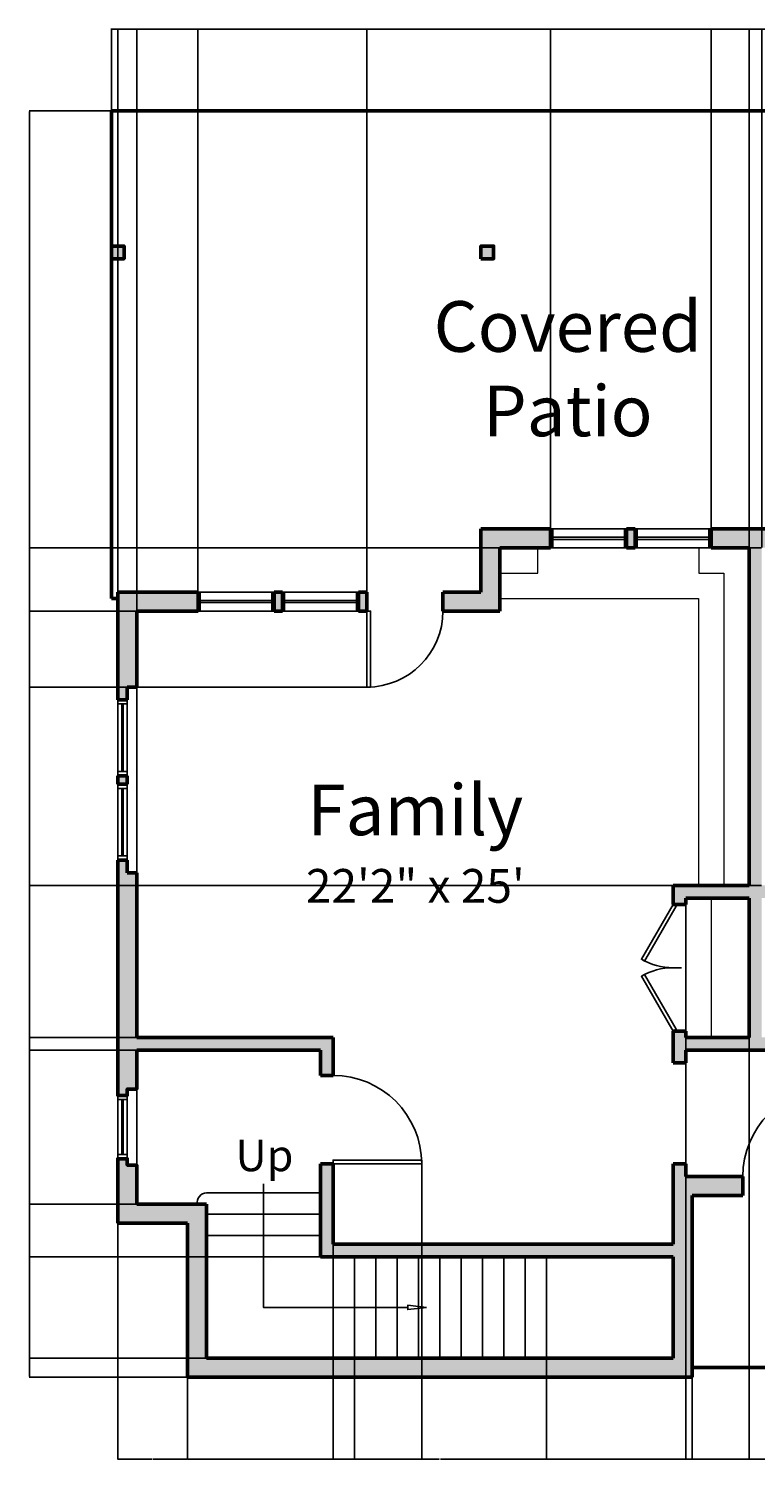
# Model space of a CAD drawing. Units: inches. Extents: x 296 to 2116, y 330 to 1460.
# Tile 7 of 9: x 1276 to 1620, y 779 to 1457. Entities that reach past the tile are written whole.
import ezdxf

# ---------------------------------------------------------------- set-up
doc = ezdxf.new("R2010")
doc.units = ezdxf.units.IN
for name, color, linetype, lineweight in [('A-ANNO-DIMS', 2, 'Continuous', 18), ('A-ANNO-TEXT', 7, 'Continuous', 18), ('A-AREA-IDEN', 7, 'Continuous', 25), ('A-DOOR', 3, 'Continuous', 25), ('A-FLOR-FIXT', 8, 'Continuous', 18), ('A-FLOR-STRS', 40, 'Continuous', 25), ('A-GLAZ', 4, 'Continuous', 25), ('A-WALL', 7, 'Continuous', 50), ('A-WALL-PATT', 8, 'Continuous', 13)]:
    doc.layers.add(name, color=color, linetype=linetype, lineweight=lineweight)
doc.styles.get("Standard").update_dxf_attribs({"font": 'arial.ttf'})
doc.dimstyles.get("Standard").update_dxf_attribs({"dimtxt": 0.18, "dimasz": 0.18, "dimexe": 0.18, "dimexo": 0.0625, "dimgap": 0.09, "dimtad": 0, "dimtih": 1, "dimtoh": 1, "dimdec": 4, "dimzin": 0, "dimdsep": 46, "dimtxsty": 'Standard', "dimcen": 0.09, "dimadec": 0, "dimazin": 0, "dimtfac": 1, "dimtdec": 4, "dimtofl": 0, "dimtmove": 0, "dimatfit": 3, "dimfxl": 1, "dimtolj": 1, "dimtzin": 0, "dimarcsym": 0})

# ---------------------------------------------------------------- blocks, each defined once
blk = doc.blocks.new('*U22')
for p, q in [((0, 0), (0, 4)), ((36, 0), (36, 4))]:
    blk.add_line(p, q)
blk.add_lwpolyline([(0, 0), (0, -36), (1.75, -36), (1.75, 0)], close=True)
blk.add_arc((0, 0), 36, 270, 0)
blk = doc.blocks.new('*U23')
for p, q in [((-40, 0), (-40, -4)), ((0, 0), (0, -4))]:
    blk.add_line(p, q)
blk.add_lwpolyline([(0, 0), (0, 40), (-1.75, 40), (-1.75, 0)], close=True)
blk.add_arc((0, 0), 40, 90, 180)
blk = doc.blocks.new('*U26')
for p, q in [((-30, 0), (-30, 4)), ((0, 0), (0, 4))]:
    blk.add_line(p, q)
blk.add_lwpolyline([(0, 0), (-25.98, -15), (-26.86, -13.48), (-0.88, 1.52)], close=True)
blk.add_arc((0, 0), 30, 180, 210)
blk = doc.blocks.new('*D67')
at = {"layer": 'A-ANNO-DIMS', "color": 0, "lineweight": -2, "transparency": 16777216}
for p, q in [((1315.18, 1418.02), (1315.18, 1456.98)), ((1315.36, 1456.8), (1695.9, 1456.8)), ((2077, 1456.8), (1696.47, 1456.8)), ((2077.18, 1408.02), (2077.18, 1456.98))]:
    blk.add_line(p, q, dxfattribs=at)
at = {"layer": 'A-ANNO-DIMS', "color": 0, "transparency": 16777216}
for points in [[(1315.36, 1456.83), (1315.36, 1456.77), (1315.18, 1456.8)], [(2077, 1456.83), (2077, 1456.77), (2077.18, 1456.8)]]:
    blk.add_solid(points, dxfattribs=at)
at = {"layer": 'Defpoints', "color": 0, "transparency": 16777216}
for p in [(2077.18, 1456.8), (1315.18, 1417.95), (2077.18, 1407.95)]:
    blk.add_point(p, dxfattribs=at)
at = {"layer": 'A-ANNO-DIMS', "color": 0, "transparency": 16777216, "insert": (1696.18, 1456.8), "char_height": 0.18, "attachment_point": 5}
blk.add_mtext('\\A1;762', dxfattribs=at)
blk = doc.blocks.new('*D68')
at = {"layer": 'A-ANNO-DIMS', "color": 0, "lineweight": -2, "transparency": 16777216}
for p, q in [((1315.12, 1417.95), (1276.15, 1417.95)), ((1276.33, 1417.77), (1276.33, 1118.16)), ((1276.33, 818.18), (1276.33, 1117.79)), ((1351.12, 818), (1276.15, 818))]:
    blk.add_line(p, q, dxfattribs=at)
at = {"layer": 'A-ANNO-DIMS', "color": 0, "transparency": 16777216}
for points in [[(1276.3, 1417.77), (1276.36, 1417.77), (1276.33, 1417.95)], [(1276.3, 818.18), (1276.36, 818.18), (1276.33, 818)]]:
    blk.add_solid(points, dxfattribs=at)
at = {"layer": 'Defpoints', "color": 0, "transparency": 16777216}
for p in [(1276.33, 1417.95), (1315.18, 1417.95), (1351.18, 818)]:
    blk.add_point(p, dxfattribs=at)
at = {"layer": 'A-ANNO-DIMS', "color": 0, "transparency": 16777216, "insert": (1276.33, 1117.98), "char_height": 0.18, "attachment_point": 5}
blk.add_mtext('\\A1;600', dxfattribs=at)
blk = doc.blocks.new('*D69')
at = {"layer": 'A-ANNO-DIMS', "color": 0, "lineweight": -2, "transparency": 16777216}
for p, q in [((1318.18, 1189.89), (1318.18, 778.97)), ((1351.18, 817.94), (1351.18, 778.97)), ((1318.36, 779.15), (1334.46, 779.15)), ((1351, 779.15), (1334.9, 779.15))]:
    blk.add_line(p, q, dxfattribs=at)
at = {"layer": 'A-ANNO-DIMS', "color": 0, "transparency": 16777216}
for points in [[(1318.36, 779.18), (1318.36, 779.12), (1318.18, 779.15)], [(1351, 779.18), (1351, 779.12), (1351.18, 779.15)]]:
    blk.add_solid(points, dxfattribs=at)
at = {"layer": 'Defpoints', "color": 0, "transparency": 16777216}
for p in [(1318.18, 1189.95), (1351.18, 818), (1351.18, 779.15)]:
    blk.add_point(p, dxfattribs=at)
at = {"layer": 'A-ANNO-DIMS', "color": 0, "transparency": 16777216, "insert": (1334.68, 779.15), "char_height": 0.18, "attachment_point": 5}
blk.add_mtext('\\A1;33', dxfattribs=at)
blk = doc.blocks.new('*D70')
at = {"layer": 'A-ANNO-DIMS', "color": 0, "lineweight": -2, "transparency": 16777216}
for p, q in [((1351.18, 817.94), (1351.18, 778.97)), ((1590.18, 817.94), (1590.18, 778.97)), ((1351.36, 779.15), (1470.39, 779.15)), ((1590, 779.15), (1470.97, 779.15))]:
    blk.add_line(p, q, dxfattribs=at)
at = {"layer": 'A-ANNO-DIMS', "color": 0, "transparency": 16777216}
for points in [[(1351.36, 779.18), (1351.36, 779.12), (1351.18, 779.15)], [(1590, 779.18), (1590, 779.12), (1590.18, 779.15)]]:
    blk.add_solid(points, dxfattribs=at)
at = {"layer": 'Defpoints', "color": 0, "transparency": 16777216}
for p in [(1351.18, 818), (1590.18, 818), (1590.18, 779.15)]:
    blk.add_point(p, dxfattribs=at)
at = {"layer": 'A-ANNO-DIMS', "color": 0, "transparency": 16777216, "insert": (1470.68, 779.15), "char_height": 0.18, "attachment_point": 5}
blk.add_mtext('\\A1;239', dxfattribs=at)
blk = doc.blocks.new('*D71')
at = {"layer": 'A-ANNO-DIMS', "color": 0, "lineweight": -2, "transparency": 16777216}
for p, q in [((1590.18, 822.44), (1590.18, 778.97)), ((1774.45, 822.44), (1774.45, 778.97)), ((1590.36, 779.15), (1681.86, 779.15)), ((1774.27, 779.15), (1682.77, 779.15))]:
    blk.add_line(p, q, dxfattribs=at)
at = {"layer": 'A-ANNO-DIMS', "color": 0, "transparency": 16777216}
for points in [[(1590.36, 779.18), (1590.36, 779.12), (1590.18, 779.15)], [(1774.27, 779.18), (1774.27, 779.12), (1774.45, 779.15)]]:
    blk.add_solid(points, dxfattribs=at)
at = {"layer": 'Defpoints', "color": 0, "transparency": 16777216}
for p in [(1590.18, 822.5), (1774.45, 822.5), (1774.45, 779.15)]:
    blk.add_point(p, dxfattribs=at)
at = {"layer": 'A-ANNO-DIMS', "color": 0, "transparency": 16777216, "insert": (1682.31, 779.15), "char_height": 0.18, "attachment_point": 5}
blk.add_mtext('\\A1;184.26', dxfattribs=at)
blk = doc.blocks.new('*D107')
at = {"layer": 'A-ANNO-DIMS', "color": 0, "lineweight": -2, "transparency": 16777216}
for p, q in [((1318.18, 1190.02), (1318.18, 1456.98)), ((1318.36, 1456.8), (1467.22, 1456.8)), ((1617, 1456.8), (1468.15, 1456.8)), ((1617.18, 1211.02), (1617.18, 1456.98))]:
    blk.add_line(p, q, dxfattribs=at)
at = {"layer": 'A-ANNO-DIMS', "color": 0, "transparency": 16777216}
for points in [[(1318.36, 1456.83), (1318.36, 1456.77), (1318.18, 1456.8)], [(1617, 1456.83), (1617, 1456.77), (1617.18, 1456.8)]]:
    blk.add_solid(points, dxfattribs=at)
at = {"layer": 'Defpoints', "color": 0, "transparency": 16777216}
for p in [(1617.18, 1456.8), (1617.18, 1210.95), (1318.18, 1189.95)]:
    blk.add_point(p, dxfattribs=at)
at = {"layer": 'A-ANNO-DIMS', "color": 0, "transparency": 16777216, "insert": (1467.68, 1456.8), "char_height": 0.18, "attachment_point": 5}
blk.add_mtext('\\A1;299.00', dxfattribs=at)
blk = doc.blocks.new('*D108')
at = {"layer": 'A-ANNO-DIMS', "color": 0, "lineweight": -2, "transparency": 16777216}
for p, q in [((1617.18, 1211.02), (1617.18, 1456.98)), ((1617.36, 1456.8), (1619.86, 1456.8)), ((1623, 1456.8), (1620.51, 1456.8)), ((1623.18, 1211.02), (1623.18, 1456.98))]:
    blk.add_line(p, q, dxfattribs=at)
at = {"layer": 'A-ANNO-DIMS', "color": 0, "transparency": 16777216}
for points in [[(1617.36, 1456.83), (1617.36, 1456.77), (1617.18, 1456.8)], [(1623, 1456.83), (1623, 1456.77), (1623.18, 1456.8)]]:
    blk.add_solid(points, dxfattribs=at)
at = {"layer": 'Defpoints', "color": 0, "transparency": 16777216}
for p in [(1623.18, 1456.8), (1617.18, 1210.95), (1623.18, 1210.95)]:
    blk.add_point(p, dxfattribs=at)
at = {"layer": 'A-ANNO-DIMS', "color": 0, "transparency": 16777216, "insert": (1620.18, 1456.8), "char_height": 0.18, "attachment_point": 5}
blk.add_mtext('\\A1;6.00', dxfattribs=at)
blk = doc.blocks.new('*D111')
at = {"layer": 'A-ANNO-DIMS', "color": 0, "lineweight": -2, "transparency": 16777216}
for p, q in [((1318.18, 1190.02), (1318.18, 1456.98)), ((1318.36, 1456.8), (1322.36, 1456.8)), ((1327, 1456.8), (1323.01, 1456.8)), ((1327.18, 1181.02), (1327.18, 1456.98))]:
    blk.add_line(p, q, dxfattribs=at)
at = {"layer": 'A-ANNO-DIMS', "color": 0, "transparency": 16777216}
for points in [[(1318.36, 1456.83), (1318.36, 1456.77), (1318.18, 1456.8)], [(1327, 1456.83), (1327, 1456.77), (1327.18, 1456.8)]]:
    blk.add_solid(points, dxfattribs=at)
at = {"layer": 'Defpoints', "color": 0, "transparency": 16777216}
for p in [(1327.18, 1456.8), (1318.18, 1189.95), (1327.18, 1180.95)]:
    blk.add_point(p, dxfattribs=at)
at = {"layer": 'A-ANNO-DIMS', "color": 0, "transparency": 16777216, "insert": (1322.68, 1456.8), "char_height": 0.18, "attachment_point": 5}
blk.add_mtext('\\A1;9.00', dxfattribs=at)
blk = doc.blocks.new('*D112')
at = {"layer": 'A-ANNO-DIMS', "color": 0, "lineweight": -2, "transparency": 16777216}
for p, q in [((1327.12, 1180.95), (1276.15, 1180.95)), ((1276.33, 1180.77), (1276.33, 1080.14)), ((1276.33, 979.13), (1276.33, 1079.77)), ((1327.12, 978.95), (1276.15, 978.95))]:
    blk.add_line(p, q, dxfattribs=at)
at = {"layer": 'A-ANNO-DIMS', "color": 0, "transparency": 16777216}
for points in [[(1276.3, 1180.77), (1276.36, 1180.77), (1276.33, 1180.95)], [(1276.3, 979.13), (1276.36, 979.13), (1276.33, 978.95)]]:
    blk.add_solid(points, dxfattribs=at)
at = {"layer": 'Defpoints', "color": 0, "transparency": 16777216}
for p in [(1276.33, 1180.95), (1327.18, 1180.95), (1327.18, 978.95)]:
    blk.add_point(p, dxfattribs=at)
at = {"layer": 'A-ANNO-DIMS', "color": 0, "transparency": 16777216, "insert": (1276.33, 1079.95), "char_height": 0.18, "attachment_point": 5}
blk.add_mtext('\\A1;202.00', dxfattribs=at)
blk = doc.blocks.new('*D113')
at = {"layer": 'A-ANNO-DIMS', "color": 0, "lineweight": -2, "transparency": 16777216}
for p, q in [((1327.12, 972.95), (1276.15, 972.95)), ((1276.33, 972.77), (1276.33, 936.64)), ((1276.33, 900.13), (1276.33, 936.27)), ((1327.12, 899.95), (1276.15, 899.95))]:
    blk.add_line(p, q, dxfattribs=at)
at = {"layer": 'A-ANNO-DIMS', "color": 0, "transparency": 16777216}
for points in [[(1276.3, 972.77), (1276.36, 972.77), (1276.33, 972.95)], [(1276.3, 900.13), (1276.36, 900.13), (1276.33, 899.95)]]:
    blk.add_solid(points, dxfattribs=at)
at = {"layer": 'Defpoints', "color": 0, "transparency": 16777216}
for p in [(1327.18, 972.95), (1276.33, 899.95), (1327.18, 899.95)]:
    blk.add_point(p, dxfattribs=at)
at = {"layer": 'A-ANNO-DIMS', "color": 0, "transparency": 16777216, "insert": (1276.33, 936.45), "char_height": 0.18, "attachment_point": 5}
blk.add_mtext('\\A1;73.00', dxfattribs=at)
blk = doc.blocks.new('*D114')
at = {"layer": 'A-ANNO-DIMS', "color": 0, "lineweight": -2, "transparency": 16777216}
for p, q in [((1581.12, 875), (1276.15, 875)), ((1276.33, 874.82), (1276.33, 851.18)), ((1276.33, 827.18), (1276.33, 850.82)), ((1581.12, 827), (1276.15, 827))]:
    blk.add_line(p, q, dxfattribs=at)
at = {"layer": 'A-ANNO-DIMS', "color": 0, "transparency": 16777216}
for points in [[(1276.3, 874.82), (1276.36, 874.82), (1276.33, 875)], [(1276.3, 827.18), (1276.36, 827.18), (1276.33, 827)]]:
    blk.add_solid(points, dxfattribs=at)
at = {"layer": 'Defpoints', "color": 0, "transparency": 16777216}
for p in [(1581.18, 875), (1276.33, 827), (1581.18, 827)]:
    blk.add_point(p, dxfattribs=at)
at = {"layer": 'A-ANNO-DIMS', "color": 0, "transparency": 16777216, "insert": (1276.33, 851), "char_height": 0.18, "attachment_point": 5}
blk.add_mtext('\\A1;48.00', dxfattribs=at)
blk = doc.blocks.new('*D115')
at = {"layer": 'A-ANNO-DIMS', "color": 0, "lineweight": -2, "transparency": 16777216}
for p, q in [((1420.18, 874.94), (1420.18, 778.97)), ((1430.28, 874.94), (1430.28, 778.97)), ((1420.36, 779.15), (1424.85, 779.15)), ((1430.1, 779.15), (1425.62, 779.15))]:
    blk.add_line(p, q, dxfattribs=at)
at = {"layer": 'A-ANNO-DIMS', "color": 0, "transparency": 16777216}
for points in [[(1420.36, 779.18), (1420.36, 779.12), (1420.18, 779.15)], [(1430.1, 779.18), (1430.1, 779.12), (1430.28, 779.15)]]:
    blk.add_solid(points, dxfattribs=at)
at = {"layer": 'Defpoints', "color": 0, "transparency": 16777216}
for p in [(1420.18, 875), (1430.28, 875), (1430.28, 779.15)]:
    blk.add_point(p, dxfattribs=at)
at = {"layer": 'A-ANNO-DIMS', "color": 0, "transparency": 16777216, "insert": (1425.23, 779.15), "char_height": 0.18, "attachment_point": 5}
blk.add_mtext('\\A1;10.10', dxfattribs=at)
blk = doc.blocks.new('*D116')
at = {"layer": 'A-ANNO-DIMS', "color": 0, "lineweight": -2, "transparency": 16777216}
for p, q in [((1420.18, 826.94), (1420.18, 778.97)), ((1521.18, 826.94), (1521.18, 778.97)), ((1420.36, 779.15), (1470.23, 779.15)), ((1521, 779.15), (1471.14, 779.15))]:
    blk.add_line(p, q, dxfattribs=at)
at = {"layer": 'A-ANNO-DIMS', "color": 0, "transparency": 16777216}
for points in [[(1420.36, 779.18), (1420.36, 779.12), (1420.18, 779.15)], [(1521, 779.18), (1521, 779.12), (1521.18, 779.15)]]:
    blk.add_solid(points, dxfattribs=at)
at = {"layer": 'Defpoints', "color": 0, "transparency": 16777216}
for p in [(1420.18, 827), (1521.18, 827), (1521.18, 779.15)]:
    blk.add_point(p, dxfattribs=at)
at = {"layer": 'A-ANNO-DIMS', "color": 0, "transparency": 16777216, "insert": (1470.68, 779.15), "char_height": 0.18, "attachment_point": 5}
blk.add_mtext('\\A1;101.00', dxfattribs=at)
blk = doc.blocks.new('*D117')
at = {"layer": 'A-ANNO-DIMS', "color": 0, "lineweight": -2, "transparency": 16777216}
for p, q in [((1587.18, 1044.89), (1587.18, 778.97)), ((1617.18, 1044.89), (1617.18, 778.97)), ((1587.36, 779.15), (1601.79, 779.15)), ((1617, 779.15), (1602.58, 779.15))]:
    blk.add_line(p, q, dxfattribs=at)
at = {"layer": 'A-ANNO-DIMS', "color": 0, "transparency": 16777216}
for points in [[(1587.36, 779.18), (1587.36, 779.12), (1587.18, 779.15)], [(1617, 779.18), (1617, 779.12), (1617.18, 779.15)]]:
    blk.add_solid(points, dxfattribs=at)
at = {"layer": 'Defpoints', "color": 0, "transparency": 16777216}
for p in [(1587.18, 1044.95), (1617.18, 1044.95), (1617.18, 779.15)]:
    blk.add_point(p, dxfattribs=at)
at = {"layer": 'A-ANNO-DIMS', "color": 0, "transparency": 16777216, "insert": (1602.18, 779.15), "char_height": 0.18, "attachment_point": 5}
blk.add_mtext('\\A1;30.00', dxfattribs=at)
blk = doc.blocks.new('*D118')
at = {"layer": 'A-ANNO-DIMS', "color": 0, "lineweight": -2, "transparency": 16777216}
for p, q in [((1623.12, 1210.95), (1276.15, 1210.95)), ((1276.33, 1210.77), (1276.33, 1131.14)), ((1276.33, 1051.13), (1276.33, 1130.77)), ((1623.12, 1050.95), (1276.15, 1050.95))]:
    blk.add_line(p, q, dxfattribs=at)
at = {"layer": 'A-ANNO-DIMS', "color": 0, "transparency": 16777216}
for points in [[(1276.3, 1210.77), (1276.36, 1210.77), (1276.33, 1210.95)], [(1276.3, 1051.13), (1276.36, 1051.13), (1276.33, 1050.95)]]:
    blk.add_solid(points, dxfattribs=at)
at = {"layer": 'Defpoints', "color": 0, "transparency": 16777216}
for p in [(1276.33, 1210.95), (1623.18, 1210.95), (1623.18, 1050.95)]:
    blk.add_point(p, dxfattribs=at)
at = {"layer": 'A-ANNO-DIMS', "color": 0, "transparency": 16777216, "insert": (1276.33, 1130.95), "char_height": 0.18, "attachment_point": 5}
blk.add_mtext('\\A1;160.00', dxfattribs=at)
blk = doc.blocks.new('*D126')
at = {"layer": 'A-ANNO-DIMS', "color": 0, "lineweight": -2, "transparency": 16777216}
for p, q in [((1436.12, 1180.95), (1276.15, 1180.95)), ((1276.33, 1180.77), (1276.33, 1163.14)), ((1276.33, 1145.13), (1276.33, 1162.77)), ((1436.12, 1144.95), (1276.15, 1144.95))]:
    blk.add_line(p, q, dxfattribs=at)
at = {"layer": 'A-ANNO-DIMS', "color": 0, "transparency": 16777216}
for points in [[(1276.3, 1180.77), (1276.36, 1180.77), (1276.33, 1180.95)], [(1276.3, 1145.13), (1276.36, 1145.13), (1276.33, 1144.95)]]:
    blk.add_solid(points, dxfattribs=at)
at = {"layer": 'Defpoints', "color": 0, "transparency": 16777216}
for p in [(1436.18, 1180.95), (1276.33, 1144.95), (1436.18, 1144.95)]:
    blk.add_point(p, dxfattribs=at)
at = {"layer": 'A-ANNO-DIMS', "color": 0, "transparency": 16777216, "insert": (1276.33, 1162.95), "char_height": 0.18, "attachment_point": 5}
blk.add_mtext('\\A1;36.00', dxfattribs=at)
blk = doc.blocks.new('*D127')
at = {"layer": 'A-ANNO-DIMS', "color": 0, "lineweight": -2, "transparency": 16777216}
for p, q in [((1420.13, 920.73), (1420.13, 778.97)), ((1462.13, 920.73), (1462.13, 778.97)), ((1420.31, 779.15), (1440.74, 779.15)), ((1461.95, 779.15), (1441.53, 779.15))]:
    blk.add_line(p, q, dxfattribs=at)
at = {"layer": 'A-ANNO-DIMS', "color": 0, "transparency": 16777216}
for points in [[(1420.31, 779.18), (1420.31, 779.12), (1420.13, 779.15)], [(1461.95, 779.18), (1461.95, 779.12), (1462.13, 779.15)]]:
    blk.add_solid(points, dxfattribs=at)
at = {"layer": 'Defpoints', "color": 0, "transparency": 16777216}
for p in [(1420.13, 920.79), (1462.13, 920.79), (1462.13, 779.15)]:
    blk.add_point(p, dxfattribs=at)
at = {"layer": 'A-ANNO-DIMS', "color": 0, "transparency": 16777216, "insert": (1441.13, 779.15), "char_height": 0.18, "attachment_point": 5}
blk.add_mtext('\\A1;42.00', dxfattribs=at)
blk = doc.blocks.new('*D129')
at = {"layer": 'A-ANNO-DIMS', "color": 0, "lineweight": -2, "transparency": 16777216}
for p, q in [((1356.18, 1190.02), (1356.18, 1456.98)), ((1356.36, 1456.8), (1395.79, 1456.8)), ((1436, 1456.8), (1396.58, 1456.8)), ((1436.18, 1190.02), (1436.18, 1456.98))]:
    blk.add_line(p, q, dxfattribs=at)
at = {"layer": 'A-ANNO-DIMS', "color": 0, "transparency": 16777216}
for points in [[(1356.36, 1456.83), (1356.36, 1456.77), (1356.18, 1456.8)], [(1436, 1456.83), (1436, 1456.77), (1436.18, 1456.8)]]:
    blk.add_solid(points, dxfattribs=at)
at = {"layer": 'Defpoints', "color": 0, "transparency": 16777216}
for p in [(1436.18, 1456.8), (1356.18, 1189.95), (1436.18, 1189.95)]:
    blk.add_point(p, dxfattribs=at)
at = {"layer": 'A-ANNO-DIMS', "color": 0, "transparency": 16777216, "insert": (1396.18, 1456.8), "char_height": 0.18, "attachment_point": 5}
blk.add_mtext('\\A1;80.00', dxfattribs=at)
blk = doc.blocks.new('*D130')
at = {"layer": 'A-ANNO-DIMS', "color": 0, "lineweight": -2, "transparency": 16777216}
for p, q in [((1523.18, 1220.02), (1523.18, 1456.98)), ((1523.36, 1456.8), (1560.79, 1456.8)), ((1599, 1456.8), (1561.58, 1456.8)), ((1599.18, 1220.02), (1599.18, 1456.98))]:
    blk.add_line(p, q, dxfattribs=at)
at = {"layer": 'A-ANNO-DIMS', "color": 0, "transparency": 16777216}
for points in [[(1523.36, 1456.83), (1523.36, 1456.77), (1523.18, 1456.8)], [(1599, 1456.83), (1599, 1456.77), (1599.18, 1456.8)]]:
    blk.add_solid(points, dxfattribs=at)
at = {"layer": 'Defpoints', "color": 0, "transparency": 16777216}
for p in [(1599.18, 1456.8), (1523.18, 1219.95), (1599.18, 1219.95)]:
    blk.add_point(p, dxfattribs=at)
at = {"layer": 'A-ANNO-DIMS', "color": 0, "transparency": 16777216, "insert": (1561.18, 1456.8), "char_height": 0.18, "attachment_point": 5}
blk.add_mtext('\\A1;76.00', dxfattribs=at)

msp = doc.modelspace()

# ---------------------------------------------------------------- hatches: boundary and pattern name
at = {"layer": 'A-WALL-PATT'}
h = msp.add_hatch(color=256, dxfattribs=at)
h.dxf.hatch_style = 1
h.paths.add_polyline_path([(1321.1832, 1353.9541), (1315.1832, 1353.9541), (1315.1832, 1347.9541), (1321.1832, 1347.9541)])
h.paths.add_polyline_path([(1496.1832, 1353.9541), (1490.1832, 1353.9541), (1490.1832, 1347.9541), (1496.1832, 1347.9541)])
h.paths.add_polyline_path([(1396.1832, 1189.9541), (1392.1832, 1189.9541), (1392.1832, 1180.9541), (1396.1832, 1180.9541)])
h.paths.add_polyline_path([(1436.1832, 1189.9541), (1432.1832, 1189.9541), (1432.1832, 1180.9541), (1436.1832, 1180.9541), (1436.1832, 1184.9541)])
h.paths.add_polyline_path([(1356.1832, 1189.9541), (1318.1832, 1189.9541), (1318.1832, 1138.9541), (1322.6832, 1138.9541), (1322.6832, 1144.9541), (1327.1832, 1144.9541), (1327.1832, 1180.9541), (1356.1832, 1180.9541)])
h.paths.add_polyline_path([(1499.1832, 1210.9541), (1523.1832, 1210.9541), (1523.1832, 1219.9541), (1490.1832, 1219.9541), (1490.1832, 1189.9541), (1472.1832, 1189.9541), (1472.1832, 1180.9541), (1499.1832, 1180.9541)])
h.paths.add_polyline_path([(1635.1832, 1219.9541), (1599.1832, 1219.9541), (1599.1832, 1210.9541), (1617.1832, 1210.9541), (1617.1832, 1050.9541), (1581.1832, 1050.9541), (1581.1832, 1041.9541), (1587.1832, 1041.9541), (1587.1832, 1044.9541), (1617.1832, 1044.9541), (1617.1832, 978.9541), (1587.1832, 978.9541), (1587.1832, 981.9541), (1581.1832, 981.9541), (1581.1832, 966.9541), (1587.1832, 966.9541), (1587.1832, 972.9541), (1773.1832, 972.9541), (1773.1832, 981.9541), (1767.1832, 981.9541), (1767.1832, 978.9541), (1733.1832, 978.9541), (1733.1832, 1044.9541), (1767.1832, 1044.9541), (1767.1832, 1041.9541), (1773.1832, 1041.9541), (1773.1832, 1056.9541), (1767.1832, 1056.9541), (1767.1832, 1050.9541), (1705.1832, 1050.9541), (1705.1832, 1044.9541), (1727.1832, 1044.9541), (1727.1832, 978.9541), (1623.1832, 978.9541), (1623.1832, 1044.9541), (1645.1832, 1044.9541), (1645.1832, 1050.9541), (1623.1832, 1050.9541), (1623.1832, 1210.9541), (1635.1832, 1210.9541)])
h.paths.add_polyline_path([(1773.1832, 1250.9541), (1767.1832, 1250.9541), (1767.1832, 1216.9541), (1719.1832, 1216.9541), (1719.1832, 1344.9541), (1767.1832, 1344.9541), (1767.1832, 1310.9541), (1773.1832, 1310.9541), (1773.1832, 1344.9541), (1779.1832, 1344.9541), (1779.1832, 1353.9541), (1710.1832, 1353.9541), (1710.1832, 1219.9541), (1699.1832, 1219.9541), (1699.1832, 1210.9541), (1767.1832, 1210.9541), (1767.1832, 1092.9541), (1773.1832, 1092.9541), (1773.1832, 1114.9541), (1780.6832, 1114.9541), (1780.6832, 1120.9541), (1773.1832, 1120.9541)])
h.paths.add_polyline_path([(1360.1832, 899.9541), (1327.1832, 899.9541), (1327.1832, 918.4541), (1322.6832, 918.4541), (1322.6832, 921.4541), (1318.1832, 921.4541), (1318.1832, 890.9541), (1351.1832, 890.9541), (1351.1832, 817.9991), (1590.1832, 817.9991), (1590.1832, 903.9541), (1614.1832, 903.9541), (1614.1832, 912.9541), (1587.1832, 912.9541), (1587.1832, 918.9541), (1581.1832, 918.9541), (1581.1832, 880.9991), (1420.1332, 880.9991), (1420.1332, 918.9541), (1415.9332, 918.9541), (1414.1332, 918.9541), (1414.1332, 874.9991), (1581.1832, 874.9991), (1581.1832, 826.9991), (1360.1832, 826.9991)])
h.paths.add_polyline_path([(1327.1832, 1056.9541), (1322.6832, 1056.9541), (1322.6832, 1062.9541), (1318.1832, 1062.9541), (1318.1832, 951.4541), (1322.6832, 951.4541), (1322.6832, 954.4541), (1327.1832, 954.4541), (1327.1832, 972.9541), (1414.1332, 972.9541), (1414.1332, 960.9541), (1420.1332, 960.9541), (1420.1332, 978.9541), (1327.1832, 978.9541)])
h.paths.add_polyline_path([(2023.1832, 1106.4482), (2018.6832, 1106.4482), (2018.6832, 1103.4482), (2014.1832, 1103.4482), (2014.1832, 1079.9541), (1928.1832, 1079.9541), (1928.1832, 1082.9541), (1922.1832, 1082.9541), (1922.1832, 1079.9541), (1878.1832, 1079.9541), (1878.1832, 1150.9541), (1881.1832, 1150.9541), (1881.1832, 1154.9541), (1881.1832, 1156.9541), (1830.1832, 1156.9541), (1830.1832, 1120.9541), (1822.6832, 1120.9541), (1822.6832, 1116.7541), (1822.6832, 1114.9541), (1830.1832, 1114.9541), (1830.1832, 1067.9541), (1834.1832, 1067.9541), (1836.1832, 1067.9541), (1836.1832, 1073.9541), (1839.1832, 1073.9541), (1839.1832, 1079.9541), (1836.1832, 1079.9541), (1836.1832, 1150.9541), (1872.1832, 1150.9541), (1872.1832, 1079.9541), (1869.1832, 1079.9541), (1869.1832, 1073.9541), (1905.1832, 1073.9541), (1922.1832, 1073.9541), (1922.1832, 1067.9541), (1926.1832, 1067.9541), (1928.1832, 1067.9541), (1928.1832, 1073.9541), (2014.1832, 1073.9541), (2014.1832, 1002.9541), (1970.1832, 1002.9541), (1928.1832, 1002.9541), (1928.1832, 1031.9541), (1922.1832, 1031.9541), (1922.1832, 1002.9541), (1836.1832, 1002.9541), (1836.1832, 1031.9541), (1834.1832, 1031.9541), (1830.1832, 1031.9541), (1830.1832, 978.9541), (1836.1832, 978.9541), (1836.1832, 996.9541), (2014.1832, 996.9541), (2014.1832, 912.9541), (1836.1832, 912.9541), (1836.1832, 942.9541), (1832.1832, 942.9541), (1830.1832, 942.9541), (1830.1832, 912.9541), (1656.1832, 912.9541), (1656.1832, 908.7541), (1656.1832, 903.9541), (2023.1832, 903.9541)])
h.paths.add_polyline_path([(2023.1832, 1165.9541), (1958.1832, 1165.9541), (1958.1832, 1156.9541), (2014.1832, 1156.9541), (2014.1832, 1139.4482), (2018.6832, 1139.4482), (2018.6832, 1136.4482), (2023.1832, 1136.4482), (2023.1832, 1159.9541)])
h.paths.add_polyline_path([(1934.1832, 1165.9541), (1928.1832, 1165.9541), (1928.1832, 1186.9541), (1923.6832, 1186.9541), (1923.6832, 1183.9541), (1919.1832, 1183.9541), (1919.1832, 1156.9541), (1911.1832, 1156.9541), (1911.1832, 1150.9541), (1922.1832, 1150.9541), (1922.1832, 1147.9541), (1928.1832, 1147.9541), (1928.1832, 1156.9541), (1934.1832, 1156.9541)])
h.paths.add_polyline_path([(1928.1832, 1293.9541), (1923.6832, 1293.9541), (1923.6832, 1290.9541), (1919.1832, 1290.9541), (1919.1832, 1219.9541), (1923.6832, 1219.9541), (1923.6832, 1216.9541), (1928.1832, 1216.9541)])
h.paths.add_polyline_path([(1928.1832, 1353.9541), (1854.1832, 1353.9541), (1854.1832, 1344.9541), (1919.1832, 1344.9541), (1919.1832, 1326.9541), (1923.6832, 1326.9541), (1923.6832, 1323.9541), (1928.1832, 1323.9541)])
h.paths.add_polyline_path([(1818.1832, 1353.9541), (1815.1832, 1353.9541), (1815.1832, 1344.9541), (1818.1832, 1344.9541)])
h.paths.add_polyline_path([(1563.1832, 1219.9541), (1559.1832, 1219.9541), (1559.1832, 1210.9541), (1563.1832, 1210.9541)])
h.paths.add_polyline_path([(1669.1832, 1219.9541), (1665.1832, 1219.9541), (1665.1832, 1210.9541), (1669.1832, 1210.9541)])
h.paths.add_polyline_path([(1322.6832, 1102.9541), (1318.1832, 1102.9541), (1318.1832, 1098.9541), (1322.6832, 1098.9541)])

# ---------------------------------------------------------------- linework, layer by layer
at = {"layer": 'A-FLOR-FIXT'}
for p, q in [((1517.1832, 1198.9541), (1517.1832, 1210.9541)), ((1593.3863, 1210.9541), (1593.3863, 1198.9541)), ((1499.1832, 1198.9541), (1517.1832, 1198.9541)), ((1593.3863, 1198.9541), (1605.1832, 1198.9541)), ((1605.1832, 1198.9541), (1605.1832, 1050.9541)), ((1499.1832, 1186.9541), (1593.1832, 1186.9541)), ((1593.1832, 1186.9541), (1593.1832, 1050.9541)), ((1599.1832, 1044.9541), (1599.1832, 978.9541))]:
    msp.add_line(p, q, dxfattribs=at)
at = {"layer": 'A-FLOR-STRS'}
for p, q in [((1414.1332, 905.2991), (1360.1832, 905.2991)), ((1414.1332, 895.1991), (1360.1832, 895.1991)), ((1414.1332, 885.0991), (1360.1832, 885.0991)), ((1414.1332, 874.9991), (1360.1832, 874.9991)), ((1420.1832, 874.9991), (1420.1832, 826.9991)), ((1430.2832, 874.9991), (1430.2832, 826.9991)), ((1440.3832, 874.9991), (1440.3832, 826.9991)), ((1450.4832, 874.9991), (1450.4832, 826.9991)), ((1460.5832, 874.9991), (1460.5832, 826.9991)), ((1470.6832, 874.9991), (1470.6832, 826.9991)), ((1480.7832, 874.9991), (1480.7832, 826.9991)), ((1490.8832, 874.9991), (1490.8832, 826.9991)), ((1500.9832, 874.9991), (1500.9832, 826.9991)), ((1511.0832, 874.9991), (1511.0832, 826.9991)), ((1521.1832, 874.9991), (1521.1832, 826.9991))]:
    msp.add_line(p, q, dxfattribs=at)
msp.add_lwpolyline([(1387.1582, 909.6129), (1387.1582, 850.9991), (1455.4988, 850.9991)], dxfattribs=at)
msp.add_lwpolyline([(1464.3667, 850.9991), (1455.4988, 852.0151), (1455.4988, 849.9575)], close=True, dxfattribs=at)
msp.add_arc((1360.4547, 900.6636), 4.6434, 93.351611, 188.7892, dxfattribs=at)
at = {"layer": 'A-GLAZ'}
for p, q in [((1524.1832, 1210.9541), (1524.1832, 1219.9541)), ((1524.1832, 1215.9541), (1558.1832, 1215.9541)), ((1558.1832, 1214.9541), (1524.1832, 1214.9541)), ((1558.1832, 1219.9541), (1558.1832, 1210.9541)), ((1564.1832, 1210.9541), (1564.1832, 1219.9541)), ((1564.1832, 1215.9541), (1598.1832, 1215.9541)), ((1598.1832, 1214.9541), (1564.1832, 1214.9541)), ((1598.1832, 1219.9541), (1598.1832, 1210.9541)), ((1357.1832, 1180.9541), (1357.1832, 1189.9541)), ((1391.1832, 1189.9541), (1391.1832, 1180.9541)), ((1397.1832, 1180.9541), (1397.1832, 1189.9541)), ((1431.1832, 1189.9541), (1431.1832, 1180.9541)), ((1357.1832, 1185.9541), (1391.1832, 1185.9541)), ((1391.1832, 1184.9541), (1357.1832, 1184.9541)), ((1397.1832, 1185.9541), (1431.1832, 1185.9541)), ((1431.1832, 1184.9541), (1397.1832, 1184.9541)), ((1318.1832, 1102.9541), (1318.1832, 1138.9541)), ((1318.1832, 1138.9541), (1322.6832, 1138.9541)), ((1318.1832, 1136.9541), (1322.6832, 1136.9541)), ((1320.1832, 1104.9541), (1320.1832, 1136.9541)), ((1320.6832, 1136.9541), (1320.6832, 1104.9541)), ((1322.6832, 1138.9541), (1322.6832, 1102.9541)), ((1322.6832, 1104.9541), (1318.1832, 1104.9541)), ((1322.6832, 1102.9541), (1318.1832, 1102.9541)), ((1318.1832, 1062.9541), (1318.1832, 1098.9541)), ((1318.1832, 1098.9541), (1322.6832, 1098.9541)), ((1322.6832, 1098.9541), (1322.6832, 1062.9541)), ((1318.1832, 1096.9541), (1322.6832, 1096.9541)), ((1320.1832, 1064.9541), (1320.1832, 1096.9541)), ((1320.6832, 1096.9541), (1320.6832, 1064.9541)), ((1322.6832, 1064.9541), (1318.1832, 1064.9541)), ((1322.6832, 1062.9541), (1318.1832, 1062.9541)), ((1318.1832, 949.4541), (1322.6832, 949.4541)), ((1320.1832, 923.4541), (1320.1832, 949.4541)), ((1320.6832, 949.4541), (1320.6832, 923.4541)), ((1322.6832, 923.4541), (1318.1832, 923.4541))]:
    msp.add_line(p, q, dxfattribs=at)
for points in [[(1559.1832, 1219.9541), (1559.1832, 1210.9541), (1523.1832, 1210.9541), (1523.1832, 1219.9541)], [(1599.1832, 1219.9541), (1599.1832, 1210.9541), (1563.1832, 1210.9541), (1563.1832, 1219.9541)], [(1392.1832, 1189.9541), (1392.1832, 1180.9541), (1356.1832, 1180.9541), (1356.1832, 1189.9541)], [(1432.1832, 1189.9541), (1432.1832, 1180.9541), (1396.1832, 1180.9541), (1396.1832, 1189.9541)], [(1327.1832, 1056.9541), (1322.6832, 1056.9541), (1322.6832, 1144.9541), (1327.1832, 1144.9541)], [(1318.1832, 921.4541), (1318.1832, 951.4541), (1322.6832, 951.4541), (1322.6832, 921.4541)], [(1327.1832, 918.4541), (1322.6832, 918.4541), (1322.6832, 954.4541), (1327.1832, 954.4541)]]:
    msp.add_lwpolyline(points, close=True, dxfattribs=at)
at = {"layer": 'A-WALL'}
for p, q in [((1315.1832, 1186.9541), (1315.1832, 1417.9541)), ((1315.1832, 1417.9541), (1863.1832, 1417.9541)), ((1490.1832, 1219.9541), (1523.1832, 1219.9541)), ((1490.1832, 1189.9541), (1490.1832, 1219.9541)), ((1523.1832, 1210.9541), (1523.1832, 1219.9541)), ((1559.1832, 1210.9541), (1559.1832, 1219.9541)), ((1559.1832, 1219.9541), (1563.1832, 1219.9541)), ((1563.1832, 1210.9541), (1563.1832, 1219.9541)), ((1599.1832, 1210.9541), (1599.1832, 1219.9541)), ((1599.1832, 1219.9541), (1635.1832, 1219.9541)), ((1499.1832, 1210.9541), (1523.1832, 1210.9541)), ((1499.1832, 1180.9541), (1499.1832, 1210.9541)), ((1559.1832, 1210.9541), (1563.1832, 1210.9541)), ((1599.1832, 1210.9541), (1617.1832, 1210.9541)), ((1617.1832, 1210.9541), (1617.1832, 1050.9541)), ((1315.1832, 1186.9541), (1318.1832, 1186.9541)), ((1318.1832, 1189.9541), (1318.1832, 1138.9541)), ((1318.1832, 1189.9541), (1356.1832, 1189.9541)), ((1342.1832, 1189.9541), (1356.1832, 1189.9541)), ((1356.1832, 1180.9541), (1356.1832, 1189.9541)), ((1392.1832, 1180.9541), (1392.1832, 1189.9541)), ((1392.1832, 1189.9541), (1396.1832, 1189.9541)), ((1392.1832, 1189.9541), (1396.1832, 1189.9541)), ((1396.1832, 1180.9541), (1396.1832, 1189.9541)), ((1432.1832, 1180.9541), (1432.1832, 1189.9541)), ((1432.1832, 1189.9541), (1436.1832, 1189.9541)), ((1432.1832, 1189.9541), (1436.1832, 1189.9541)), ((1436.1832, 1189.9541), (1436.1832, 1180.9541)), ((1472.1832, 1189.9541), (1472.1832, 1180.9541)), ((1472.1832, 1189.9541), (1490.1832, 1189.9541)), ((1472.1832, 1189.9541), (1490.1832, 1189.9541)), ((1327.1832, 1180.9541), (1327.1832, 1144.9541)), ((1327.1832, 1180.9541), (1356.1832, 1180.9541)), ((1392.1832, 1180.9541), (1396.1832, 1180.9541)), ((1432.1832, 1180.9541), (1436.1832, 1180.9541)), ((1472.1832, 1180.9541), (1499.1832, 1180.9541)), ((1327.1832, 1144.9541), (1322.6832, 1144.9541)), ((1322.6832, 1144.9541), (1322.6832, 1138.9541)), ((1322.6832, 1138.9541), (1318.1832, 1138.9541)), ((1322.6832, 1102.9541), (1318.1832, 1102.9541)), ((1318.1832, 1102.9541), (1318.1832, 1098.9541)), ((1322.6832, 1098.9541), (1318.1832, 1098.9541)), ((1322.6832, 1102.9541), (1322.6832, 1098.9541)), ((1322.6832, 1062.9541), (1318.1832, 1062.9541)), ((1322.6832, 1062.9541), (1322.6832, 1056.9541)), ((1327.1832, 1056.9541), (1322.6832, 1056.9541)), ((1327.1832, 1056.9541), (1327.1832, 978.9541)), ((1581.1832, 1050.9541), (1617.1832, 1050.9541)), ((1581.1832, 1050.9541), (1581.1832, 1041.9541)), ((1587.1832, 1044.9541), (1617.1832, 1044.9541)), ((1587.1832, 1044.9541), (1587.1832, 1041.9541)), ((1617.1832, 1044.9541), (1617.1832, 978.9541)), ((1581.1832, 1041.9541), (1587.1832, 1041.9541)), ((1327.1832, 978.9541), (1420.1332, 978.9541)), ((1420.1332, 978.9541), (1420.1332, 960.9541)), ((1581.1832, 981.9541), (1587.1832, 981.9541)), ((1581.1832, 981.9541), (1581.1832, 966.9541)), ((1587.1832, 981.9541), (1587.1832, 978.9541)), ((1587.1832, 978.9541), (1617.1832, 978.9541)), ((1327.1832, 972.9541), (1414.1332, 972.9541)), ((1414.1332, 972.9541), (1414.1332, 960.9541)), ((1587.1832, 972.9541), (1773.1832, 972.9541)), ((1587.1832, 972.9541), (1587.1832, 966.9541)), ((1581.1832, 966.9541), (1587.1832, 966.9541)), ((1414.1332, 960.9541), (1420.1332, 960.9541)), ((1414.1332, 918.9541), (1420.1332, 918.9541)), ((1414.1332, 918.9541), (1414.1332, 874.9991)), ((1420.1332, 918.9541), (1420.1332, 880.9991)), ((1581.1832, 918.9541), (1587.1832, 918.9541)), ((1581.1832, 918.9541), (1581.1832, 880.9991)), ((1587.1832, 918.9541), (1587.1832, 912.9541)), ((1587.1832, 912.9541), (1614.1832, 912.9541)), ((1614.1832, 903.9541), (1614.1832, 912.9541)), ((1590.1832, 903.9541), (1590.1832, 817.9991)), ((1327.1832, 899.9541), (1360.1832, 899.9541)), ((1360.1832, 899.9541), (1360.1832, 826.9991)), ((1318.1832, 890.9541), (1351.1832, 890.9541)), ((1351.1832, 890.9541), (1351.1832, 817.9991)), ((1581.1832, 874.9991), (1414.1332, 874.9991)), ((1581.1832, 880.9991), (1420.1332, 880.9991)), ((1581.1832, 874.9991), (1581.1832, 826.9991)), ((1360.1832, 826.9991), (1581.1832, 826.9991)), ((1590.1832, 822.4991), (1774.4453, 822.4991)), ((1351.1832, 817.9991), (1590.1832, 817.9991))]:
    msp.add_line(p, q, dxfattribs=at)
for points in [[(1315.1832, 1347.9541), (1321.1832, 1347.9541), (1321.1832, 1353.9541), (1315.1832, 1353.9541)], [(1490.1832, 1347.9541), (1496.1832, 1347.9541), (1496.1832, 1353.9541), (1490.1832, 1353.9541)]]:
    msp.add_lwpolyline(points, close=True, dxfattribs=at)
for points in [[(1327.1832, 972.9541), (1327.1832, 954.4541), (1322.6832, 954.4541), (1322.6832, 951.4541), (1318.1832, 951.4541), (1318.1832, 1062.9541)], [(1327.1832, 899.9541), (1327.1832, 918.4541), (1322.6832, 918.4541), (1322.6832, 921.4541), (1318.1832, 921.4541), (1318.1832, 890.9541)], [(1614.1832, 903.9541), (1590.1832, 903.9541)]]:
    msp.add_lwpolyline(points, dxfattribs=at)

# ---------------------------------------------------------------- block references
at = {"layer": 'A-DOOR'}
msp.add_blockref('*U22', (1436.1832, 1180.9541), dxfattribs=at)
at = {"layer": 'A-DOOR', "xscale": -1, "rotation": 270}
msp.add_blockref('*U26', (1581.1832, 1041.9541), dxfattribs=at)
at = {"layer": 'A-DOOR', "rotation": 270}
msp.add_blockref('*U26', (1581.1832, 981.9541), dxfattribs=at)
at = {"layer": 'A-DOOR', "xscale": 1.05, "yscale": 1.05, "zscale": 1.05, "rotation": 270}
msp.add_blockref('*U23', (1420.1332, 918.9541), dxfattribs=at)
at = {"layer": 'A-DOOR', "xscale": 1.05, "yscale": 1.05, "zscale": 1.05}
msp.add_blockref('*U23', (1656.1832, 912.9541), dxfattribs=at)

# ---------------------------------------------------------------- texts
at = {"layer": 'A-ANNO-TEXT', "insert": (1373.9428, 930.5429), "char_height": 15, "attachment_point": 1}
msp.add_mtext_dynamic_manual_height_columns('{\\fArial|b1|i0|c0|p34;Up}', width=22.506546, gutter_width=12.5, heights=[0], dxfattribs=at)
at = {"layer": 'A-AREA-IDEN', "char_height": 24, "attachment_point": 1}
for s, insert in [('\\pxqc;{\\fArial|b1|i0|c0|p34;Covered\\PPatio}', (1447.3596, 1327.8242)), ('\\pxqc;{\\fArial|b1|i0|c0|p34;Family\\P\\fArial|b0|i0|c0|p34;\\H0.66667x;22\'2" x 25\'}', (1375.1442, 1098.7394))]:
    msp.add_mtext_dynamic_manual_height_columns(s, width=167.942646, gutter_width=12.5, heights=[0], dxfattribs=dict(at, insert=insert))

# ---------------------------------------------------------------- dimensions: what is measured, and where the dimension line sits
at = {"layer": 'A-ANNO-DIMS'}
for base, p1, p2, override, picture, middle in [((2077.1832, 1456.8041), (1315.1832, 1417.9541), (2077.1832, 1407.9541), {"dimdec": 0, "dimlfac": 1, "dimrnd": 0, "dimzin": 0, "dimdsep": 46, "dimlunit": 2}, '*D67', (1696.1832, 1456.8041)), ((1617.1832, 1456.8041), (1318.1832, 1189.9541), (1617.1832, 1210.9541), {"dimdec": 2, "dimlfac": 1, "dimrnd": 0, "dimzin": 0, "dimdsep": 46, "dimlunit": 2}, '*D107', (1467.6832, 1456.8041)), ((1327.1832, 1456.8041), (1318.1832, 1189.9541), (1327.1832, 1180.9541), {"dimdec": 2, "dimlfac": 1, "dimrnd": 0, "dimzin": 0, "dimdsep": 46, "dimlunit": 2}, '*D111', (1322.6832, 1456.8041)), ((1436.1832, 1456.8041), (1356.1832, 1189.9541), (1436.1832, 1189.9541), {"dimdec": 2, "dimlfac": 1, "dimrnd": 0, "dimzin": 0, "dimdsep": 46, "dimlunit": 2}, '*D129', (1396.1832, 1456.8041)), ((1599.1832, 1456.8041), (1523.1832, 1219.9541), (1599.1832, 1219.9541), {"dimdec": 2, "dimlfac": 1, "dimrnd": 0, "dimzin": 0, "dimdsep": 46, "dimlunit": 2}, '*D130', (1561.1832, 1456.8041)), ((1623.1832, 1456.8041), (1617.1832, 1210.9541), (1623.1832, 1210.9541), {"dimdec": 2, "dimlfac": 1, "dimrnd": 0, "dimzin": 0, "dimdsep": 46, "dimlunit": 2}, '*D108', (1620.1832, 1456.8041)), ((1351.1832, 779.1491), (1318.1832, 1189.9541), (1351.1832, 817.9991), {"dimdec": 0, "dimlfac": 1, "dimrnd": 0, "dimzin": 0, "dimdsep": 46, "dimlunit": 2}, '*D69', (1334.6832, 779.1491)), ((1617.1832, 779.1491), (1587.1832, 1044.9541), (1617.1832, 1044.9541), {"dimdec": 2, "dimlfac": 1, "dimrnd": 0, "dimzin": 0, "dimdsep": 46, "dimlunit": 2}, '*D117', (1602.1832, 779.1491)), ((1462.1332, 779.1491), (1420.1332, 920.7916), (1462.1332, 920.7916), {"dimdec": 2, "dimlfac": 1, "dimrnd": 0, "dimzin": 0, "dimdsep": 46, "dimlunit": 2}, '*D127', (1441.1332, 779.1491)), ((1430.2832, 779.1491), (1420.1832, 874.9991), (1430.2832, 874.9991), {"dimdec": 2, "dimlfac": 1, "dimrnd": 0, "dimzin": 0, "dimdsep": 46, "dimlunit": 2}, '*D115', (1425.2332, 779.1491)), ((1521.1832, 779.1491), (1420.1832, 826.9991), (1521.1832, 826.9991), {"dimdec": 2, "dimlfac": 1, "dimrnd": 0, "dimzin": 0, "dimdsep": 46, "dimlunit": 2}, '*D116', (1470.6832, 779.1491)), ((1774.4453, 779.1491), (1590.1832, 822.4991), (1774.4453, 822.4991), {"dimdec": 2, "dimlfac": 1, "dimrnd": 0, "dimzin": 0, "dimdsep": 46, "dimlunit": 2}, '*D71', (1682.3143, 779.1491)), ((1590.1832, 779.1491), (1351.1832, 817.9991), (1590.1832, 817.9991), {"dimdec": 0, "dimlfac": 1, "dimrnd": 0, "dimzin": 0, "dimdsep": 46, "dimlunit": 2}, '*D70', (1470.6832, 779.1491))]:
    dim = msp.add_linear_dim(base=base, p1=p1, p2=p2, dimstyle='Standard', override=override, dxfattribs=at)
    dim.commit()
    dim.dimension.update_dxf_attribs({"geometry": picture, "text_midpoint": middle})
for base, p1, p2, override, picture, middle in [((1276.3332, 1417.9541), (1351.1832, 817.9991), (1315.1832, 1417.9541), {"dimdec": 0, "dimlfac": 1, "dimrnd": 0, "dimzin": 0, "dimdsep": 46, "dimlunit": 2}, '*D68', (1276.3332, 1117.9766)), ((1276.3332, 1210.9541), (1623.1832, 1050.9541), (1623.1832, 1210.9541), {"dimdec": 2, "dimlfac": 1, "dimrnd": 0, "dimzin": 0, "dimdsep": 46, "dimlunit": 2}, '*D118', (1276.3332, 1130.9541)), ((1276.3332, 1180.9541), (1327.1832, 978.9541), (1327.1832, 1180.9541), {"dimdec": 2, "dimlfac": 1, "dimrnd": 0, "dimzin": 0, "dimdsep": 46, "dimlunit": 2}, '*D112', (1276.3332, 1079.9541)), ((1276.3332, 1144.9541), (1436.1832, 1180.9541), (1436.1832, 1144.9541), {"dimdec": 2, "dimlfac": 1, "dimrnd": 0, "dimzin": 0, "dimdsep": 46, "dimlunit": 2}, '*D126', (1276.3332, 1162.9541)), ((1276.3332, 899.9541), (1327.1832, 972.9541), (1327.1832, 899.9541), {"dimdec": 2, "dimlfac": 1, "dimrnd": 0, "dimzin": 0, "dimdsep": 46, "dimlunit": 2}, '*D113', (1276.3332, 936.4541)), ((1276.3332, 826.9991), (1581.1832, 874.9991), (1581.1832, 826.9991), {"dimdec": 2, "dimlfac": 1, "dimrnd": 0, "dimzin": 0, "dimdsep": 46, "dimlunit": 2}, '*D114', (1276.3332, 850.9991))]:
    dim = msp.add_linear_dim(base=base, p1=p1, p2=p2, angle=90, dimstyle='Standard', override=override, dxfattribs=at)
    dim.commit()
    dim.dimension.update_dxf_attribs({"geometry": picture, "text_midpoint": middle})

doc.saveas('drawing.dxf')
